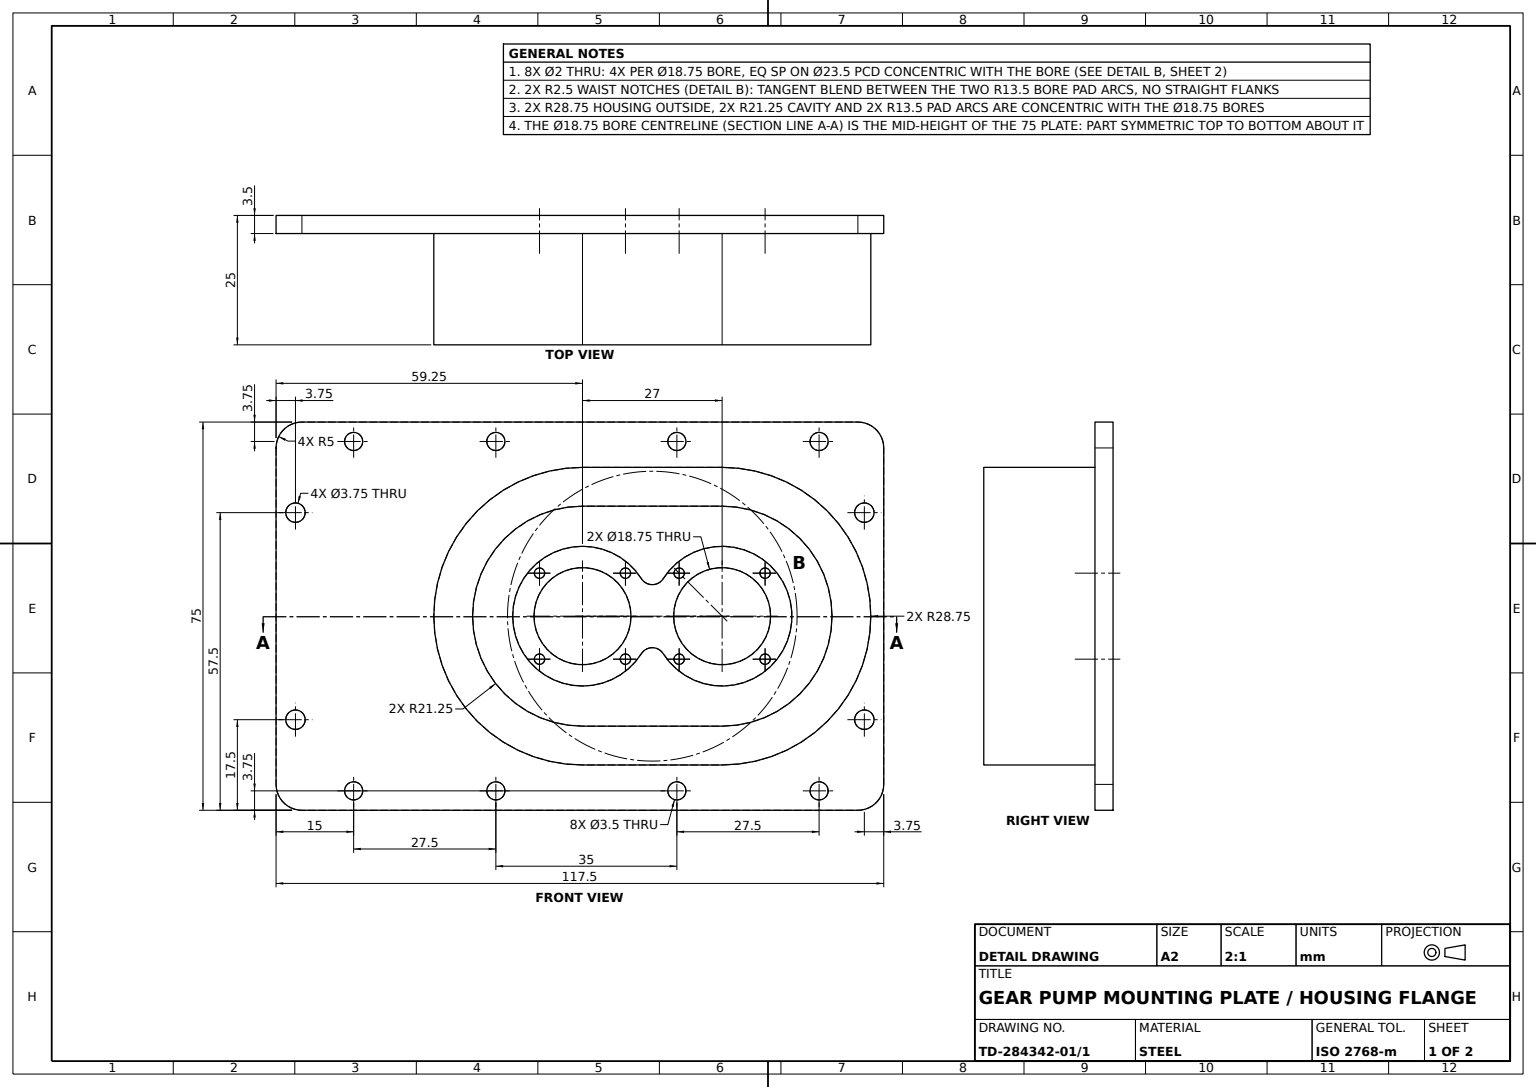
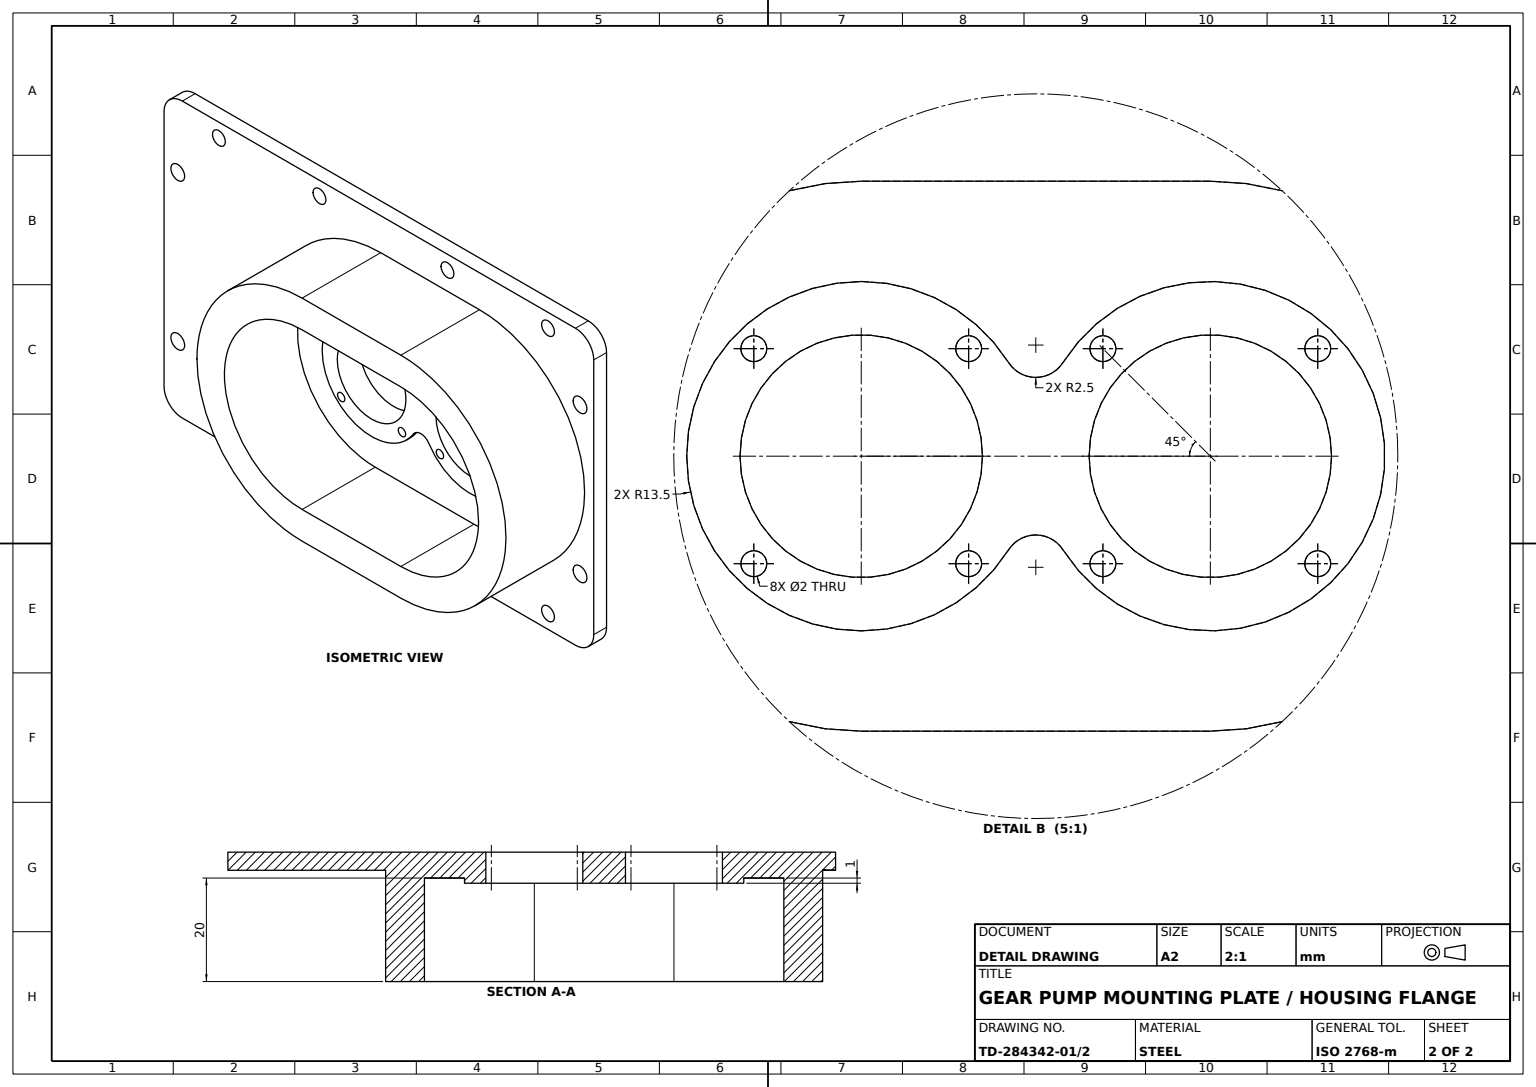
from build123d import *

# Parameters (mm, degrees)
FLANGE_PLATE_SKETCH_W              = 117.5
FLANGE_PLATE_SKETCH_H              = 75
FLANGE_PLATE_DEPTH                 = 3.5
HOUSING_WALL_DEPTH                 = 21.5
HOUSING_CAVITY_DEPTH               = 20
DUAL_BORE_SKETCH_R                 = 9.375
DUAL_BORES_DEPTH                   = 141.823471055
BORE_START                         = 1
BORE_PAD_SKETCH_R                  = 9.375
BORE_PADS_DEPTH                    = 1
BORE_SLOT_SKETCH_R                 = 1
BORE_SLOT_CUT_DEPTH                = 141.684931674
BORE_SLOT_PATTERN_4X_COUNT         = 4
BORE_NOTCH_SKETCH_R                = 1
BORE_NOTCH_CUT_DEPTH               = 141.684931674
BORE_NOTCH_PATTERN_4X_COUNT        = 4
FLANGE_CORNER_FILLETS_R5_R         = 5
FLANGE_EDGE_HOLE_SKETCH_R          = 1.75
FLANGE_EDGE_HOLE_DEPTH             = 142.044319276
FLANGE_EDGE_HOLE_PATTERN_COUNT     = 2
FLANGE_EDGE_HOLE_PATTERN_PITCH     = 27.5
FLANGE_SIDE_HOLE_SKETCH_R          = 1.75
FLANGE_SIDE_HOLES_DEPTH            = 142.044319276
FLANGE_CORNER_HOLE_SKETCH_R        = 1.875
FLANGE_CORNER_HOLES_DEPTH          = 142.044319276
FLANGE_HOLE_MIRROR_COPY_1_SKETCH_R = 1.75
FLANGE_HOLE_MIRROR_COPY_1_DEPTH    = 142.044319276


with BuildPart() as part:
    # Flange Plate Sketch → Flange Plate (new body)
    with BuildSketch(Plane.XY):
        with Locations((58.75, 37.5)):
            Rectangle(FLANGE_PLATE_SKETCH_W, FLANGE_PLATE_SKETCH_H)
    extrude(amount=FLANGE_PLATE_DEPTH)

    # Housing Wall Sketch → Housing Wall (add)
    with BuildSketch(Plane.XY.offset(3.5)):
        with BuildLine():
            Line((59.25, 66.25), (86.25, 66.25))
            ThreePointArc((86.25, 66.25), (115, 37.5), (86.25, 8.75))
            Line((86.25, 8.75), (59.25, 8.75))
            ThreePointArc((59.25, 8.75), (30.5, 37.5), (59.25, 66.25))
        make_face()
    extrude(amount=HOUSING_WALL_DEPTH)

    # Housing Cavity Sketch → Housing Cavity (cut)
    with BuildSketch(Plane.XY.offset(25)):
        with BuildLine():
            Line((86.25, 16.25), (59.25, 16.25))
            ThreePointArc((59.25, 16.25), (38, 37.5), (59.25, 58.75))
            Line((59.25, 58.75), (86.25, 58.75))
            ThreePointArc((86.25, 58.75), (107.5, 37.5), (86.25, 16.25))
        make_face()
    extrude(amount=-HOUSING_CAVITY_DEPTH, mode=Mode.SUBTRACT)

    # Dual Bore Sketch → Dual Bores (cut, through all)
    with BuildSketch(Plane.XY.offset(5)):
        with Locations((59.25, 37.5)):
            Circle(DUAL_BORE_SKETCH_R)
        with Locations((86.25, 37.5)):
            Circle(DUAL_BORE_SKETCH_R)
    extrude(amount=-DUAL_BORES_DEPTH, mode=Mode.SUBTRACT)

    # Bore Pad Sketch → Bore Pads (add)
    with BuildSketch(Plane.XY.offset(5).offset(BORE_START)):
        with BuildLine():
            ThreePointArc((70.640625, 44.745941078), (45.75, 37.5), (70.640625, 30.254058922))
            ThreePointArc((70.640625, 30.254058922), (72.75, 31.412217981), (74.859375, 30.254058922))
            ThreePointArc((74.859375, 30.254058922), (99.75, 37.5), (74.859375, 44.745941078))
            ThreePointArc((74.859375, 44.745941078), (72.75, 43.587782019), (70.640625, 44.745941078))
        make_face()
        with Locations((59.25, 37.5)):
            Circle(BORE_PAD_SKETCH_R, mode=Mode.SUBTRACT)
        with Locations((86.25, 37.5)):
            Circle(BORE_PAD_SKETCH_R, mode=Mode.SUBTRACT)
    extrude(amount=-BORE_PADS_DEPTH)

    # Bore Slot Sketch → Bore Slot Cut (cut, through all)
    with BuildSketch(Plane.XY.offset(6)):
        with Locations((67.558504679, 29.191495321)):
            Circle(BORE_SLOT_SKETCH_R)
    bore_slot_cut = extrude(amount=-BORE_SLOT_CUT_DEPTH, mode=Mode.SUBTRACT)

    # Bore Slot Pattern 4x: Bore Slot Cut ×4 about axis
    bore_slot_pattern_4x_axis = Axis((59.25, 37.5, 0), (0, 0, 1))
    for i in range(1, BORE_SLOT_PATTERN_4X_COUNT):
        add(bore_slot_cut.rotate(bore_slot_pattern_4x_axis, i * 360 / BORE_SLOT_PATTERN_4X_COUNT), mode=Mode.SUBTRACT)

    # Bore Notch Sketch → Bore Notch Cut (cut, through all)
    with BuildSketch(Plane.XY.offset(6)):
        with Locations((94.558504679, 29.191495321)):
            Circle(BORE_NOTCH_SKETCH_R)
    bore_notch_cut = extrude(amount=-BORE_NOTCH_CUT_DEPTH, mode=Mode.SUBTRACT)

    # Bore Notch Pattern 4x: Bore Notch Cut ×4 about axis
    bore_notch_pattern_4x_axis = Axis((86.25, 37.5, 0), (0, 0, 1))
    for i in range(1, BORE_NOTCH_PATTERN_4X_COUNT):
        add(bore_notch_cut.rotate(bore_notch_pattern_4x_axis, i * 360 / BORE_NOTCH_PATTERN_4X_COUNT), mode=Mode.SUBTRACT)

    # Flange Corner Fillets R5
    flange_corner_fillets_r5_edges = [part.edges().sort_by_distance(p)[0] for p in [
        (0, 75, 1.75),
        (117.5, 75, 1.75),
        (117.5, 0, 1.75),
        (0, 0, 1.75),
    ]]
    fillet(flange_corner_fillets_r5_edges, radius=FLANGE_CORNER_FILLETS_R5_R)

    # Flange Edge Hole Sketch → Flange Edge Hole (cut, through all)
    with BuildSketch(Plane.XY.offset(3.5)):
        with Locations((15, 71.25)):
            Circle(FLANGE_EDGE_HOLE_SKETCH_R)
    flange_edge_hole = extrude(amount=-FLANGE_EDGE_HOLE_DEPTH, mode=Mode.SUBTRACT)

    # Flange Edge Hole Pattern: Flange Edge Hole ×2
    with Locations(*[(i * FLANGE_EDGE_HOLE_PATTERN_PITCH, 0, 0) for i in range(1, FLANGE_EDGE_HOLE_PATTERN_COUNT)]):
        add(flange_edge_hole, mode=Mode.SUBTRACT)

    # Flange Side Hole Sketch → Flange Side Holes (cut, through all)
    with BuildSketch(Plane.XY.offset(3.5)):
        with Locations((77.5, 71.25)):
            Circle(FLANGE_SIDE_HOLE_SKETCH_R)
        with Locations((105, 71.25)):
            Circle(FLANGE_SIDE_HOLE_SKETCH_R)
    flange_side_holes = extrude(amount=-FLANGE_SIDE_HOLES_DEPTH, mode=Mode.SUBTRACT)

    # Flange Corner Hole Sketch → Flange Corner Holes (cut, through all)
    with BuildSketch(Plane.XY.offset(3.5)):
        with Locations((113.75, 57.5)):
            Circle(FLANGE_CORNER_HOLE_SKETCH_R)
        with Locations((113.75, 17.5)):
            Circle(FLANGE_CORNER_HOLE_SKETCH_R)
    flange_corner_holes = extrude(amount=-FLANGE_CORNER_HOLES_DEPTH, mode=Mode.SUBTRACT)

    # Flange Hole Mirror: Flange Edge Hole, Flange Side Holes across plane
    add(flange_edge_hole.mirror(Plane.ZX.offset(37.5)), mode=Mode.SUBTRACT)
    add(flange_side_holes.mirror(Plane.ZX.offset(37.5)), mode=Mode.SUBTRACT)

    # Flange Hole Mirror copy 1 sketch → Flange Hole Mirror copy 1 (cut, through all)
    with BuildSketch(Plane(origin=(27.5, 75, 3.5), x_dir=(1, 0, 0), z_dir=(0, 0, 1))):
        with Locations((15, -71.25)):
            Circle(FLANGE_HOLE_MIRROR_COPY_1_SKETCH_R)
    extrude(amount=-FLANGE_HOLE_MIRROR_COPY_1_DEPTH, mode=Mode.SUBTRACT)

    # Corner Hole Mirror: Flange Corner Holes across plane
    add(flange_corner_holes.mirror(Plane(origin=(58.75, 0, 0), x_dir=(0, 0, 1), z_dir=(1, 0, 0))), mode=Mode.SUBTRACT)


solid = part.part
